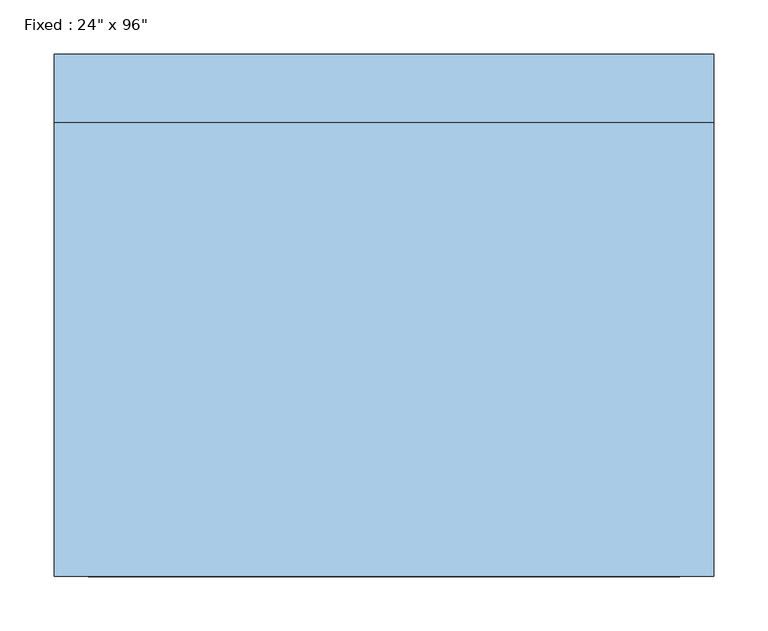
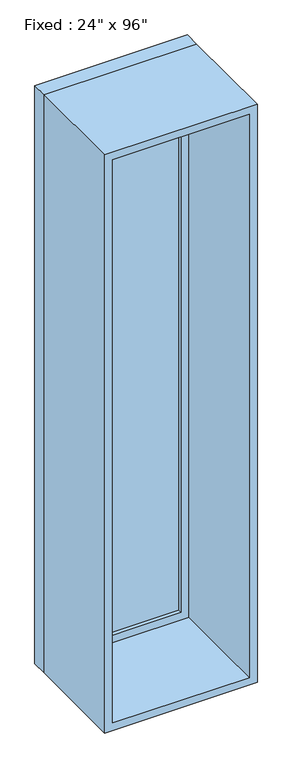
"""IFC4 building model written with IfcOpenShell, lengths in millimetres: window geometry."""

from ifc_helpers import new_model, si_unit, frame, origin, place, context, project, spatial, polyline, outline, extrude, source, transform, mapped, element, save


def window_a3455bd6(model_context):
    return source(origin(), model_context, "Body", "SweptSolid", [
        extrude(outline(polyline([(203.2, 193.5919311), (-279.4, 193.5919311), (-279.4, 206.2919311), (203.2, 206.2919311), (203.2, 193.5919311)])), frame((0.0, 0.0, 368.3), z_axis=(0.0, 0.0, 1.0), x_axis=(1.0, 0.0, 0.0)), (0.0, 0.0, 1.0), 2311.4),
        extrude(outline(polyline([(2724.15, -323.85), (323.85, -323.85), (323.85, 247.65), (2724.15, 247.65), (2724.15, -323.85)]), holes=[polyline([(2679.7, -279.4), (2679.7, 203.2), (368.3, 203.2), (368.3, -279.4), (2679.7, -279.4)])]), frame((0.0, 177.7169311, 0.0), z_axis=(0.0, 1.0, 0.0), x_axis=(0.0, 0.0, 1.0)), (0.0, 0.0, 1.0), 44.45),
        extrude(outline(polyline([(2743.2, -342.9), (304.8, -342.9), (304.8, 266.7), (2743.2, 266.7), (2743.2, -342.9)]), holes=[polyline([(2711.45, -311.15), (2711.45, 234.95), (336.55, 234.95), (336.55, -311.15), (2711.45, -311.15)])]), frame((0.0, -241.2169311, 0.0), z_axis=(0.0, 1.0, 0.0), x_axis=(0.0, 0.0, 1.0)), (0.0, 0.0, 1.0), 418.9338623),
        extrude(outline(polyline([(2743.2, 266.7), (2743.2, -342.9), (304.8, -342.9), (304.8, 266.7), (2743.2, 266.7)]), holes=[polyline([(2724.15, 247.65), (323.85, 247.65), (323.85, -323.85), (2724.15, -323.85), (2724.15, 247.65)])]), frame((0.0, 177.7169311, 0.0), z_axis=(0.0, 1.0, 0.0), x_axis=(0.0, 0.0, 1.0)), (0.0, 0.0, 1.0), 63.5),
    ])


if __name__ == "__main__":
    model = new_model("IFC4")
    model_context = context("Model", 3, world=origin())
    ifc_project = project(units=[si_unit("LENGTHUNIT", "METRE", prefix="MILLI")], contexts=[model_context])
    site = spatial("IfcSite", under=ifc_project)
    building = spatial("IfcBuilding", under=site)
    placement = place(None, origin())
    window_shape = window_a3455bd6(model_context)
    element("IfcWindow", 1, ObjectType="Fixed : 24\" x 96\"", at=placement, inside=building, context=model_context, shape_type="MappedRepresentation", body=[
        mapped(window_shape, transform((0.0, 0.0, 0.0), x_axis=(1.0, 0.0, 0.0), y_axis=(0.0, 1.0, 0.0), z_axis=(0.0, 0.0, 1.0))),
    ])
    save(model, "model.ifc")

# Revit data of these elements
# Type "Fixed : 24\" x 96\""
#   Type Mark = "6"
#   Construction Type Id = "GSP4R"
#   Assembly Code = "B2020100"
#   Analytic Construction = "1/8 in Pilkington single glazing"
#   Visual Light Transmittance = 0.9
#   Solar Heat Gain Coefficient = 0.78
#   Heat Transfer Coefficient (U) = 0.6496 BTU/(h·ft²·°F)
#   Height = 8' - 0"
#   Default Sill Height = 1' - 0"
#   Width = 2' - 0"
#   Window Inset = 0' - 0 3/4"
#   Define Thermal Properties by = 1
#   Glass Pane Material = Glass
#   Sash Material = Sash
#   Wall Closure = (empty or 0)
# Element 1 (IfcWindow, "Fixed : 24\" x 96\"")
#   Materials on its faces: "Sash", "Glass"
# Materials
#   "Glass": class "Glass", colour RGB 0 128 192, transparency 0.75, Description = "Soda Lime Glass", Cost = 0
#   "Sash": class "Wood", colour RGB 224 178 126, transparency 0
